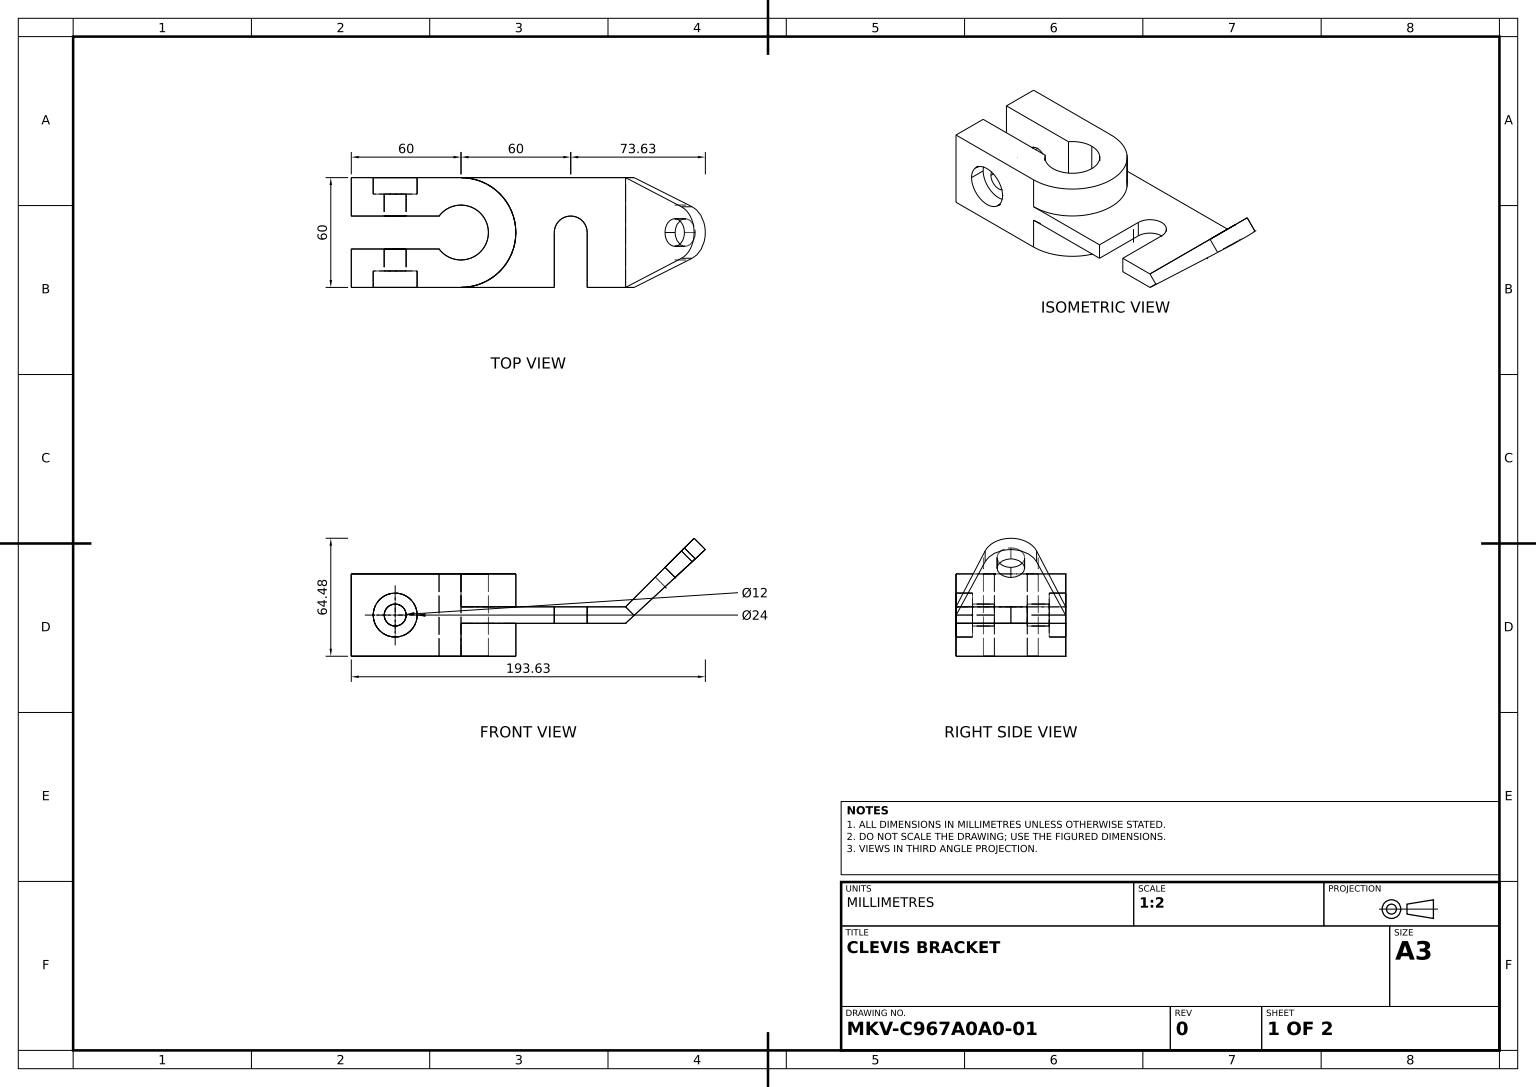
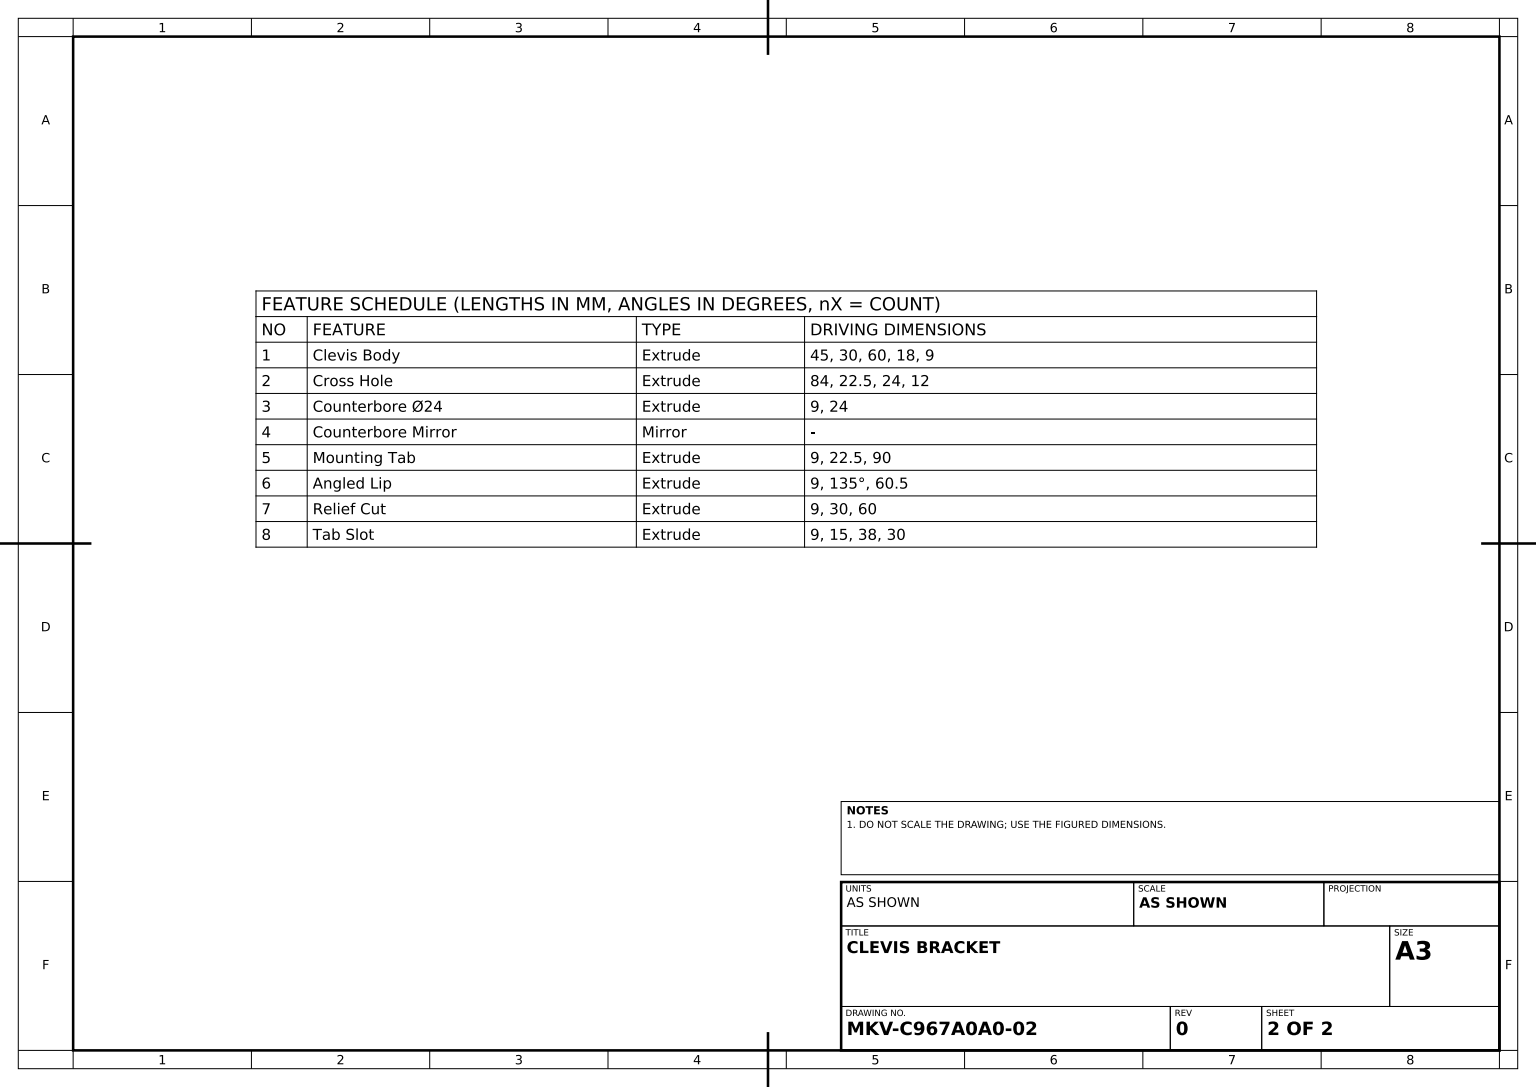
SolidWorks part; units mm, degrees
material "Plain Carbon Steel"
ref_plane "Front Plane" through (0, 0, 0) normal (0, 0, 1) x (1, 0, 0)
ref_plane "Top Plane" through (0, 0, 0) normal (0, 1, 0) x (1, 0, 0)
ref_plane "Right Plane" through (0, 0, 0) normal (1, 0, 0) x (0, 0, -1)
sketch "Clevis Body Sketch" plane through (0, 0, 0) normal (0, 1, 0) x (1, 0, 0)
  line L0 (87.3027, 0) -> (-87.3027, 0) construction
  line L1 (-12, 9) -> (-60, 9)
  line L3 (-60, -9) -> (-12, -9)
  line L4 (0, 30) -> (-60, 30)
  line L5 (-60, 30) -> (-60, 9)
  line L6 (-60, -9) -> (-60, -30)
  line L7 (-60, -30) -> (0, -30)
  arc A0 (-12, -9) -> (-12, 9) centre (0, 0) ccw
  arc A1 (0, -30) -> (0, 30) centre (0, 0) ccw
  point P6 (0, 0)
  point P12 (0, 0)
  dimension "D1" = 30
  dimension "D2" = 60
  dimension "D3" = 18
  dimension "D4" = 9
  dimension "D5" = 60
  dimension "D6" = 9
extrude "Clevis Body" add sketch "Clevis Body Sketch" along normal mid plane 45
sketch "Cross Hole Sketch" plane through (0, 0, 30) normal (0, 0, 1) x (1, 0, 0)
  line L0 (-60, -22.5) -> (0, -22.5) construction
  line L1 (-60, 22.5) -> (-60, -22.5) construction
  circle A0 centre (-36, 0) radius 6
  dimension "D3" = 12
  dimension "D1" = 22.5
  dimension "D2" = 24
extrude "Cross Hole" cut sketch "Cross Hole Sketch" against normal blind 84
sketch "Counterbore Sketch" plane through (0, 0, 30) normal (0, 0, 1) x (1, 0, 0)
  circle A0 centre (-36, 0) radius 12
  dimension "D1" = 24
extrude "Counterbore Ø24" cut sketch "Counterbore Sketch" against normal blind 9
mirror "Counterbore Mirror" about plane through (0, 0, 0) normal (0, 0, 1) of "Counterbore Ø24"
sketch "Mounting Tab Sketch" plane through (0, 22.5, 0) normal (0, 1, 0) x (1, 0, 0)
  line L0 (0, 30) -> (90, 30)
  line L1 (90, 30) -> (90, -30)
  line L2 (90, -30) -> (0, -30)
  arc A0 (0, -30) -> (0, 30) centre (0, 0) ccw construction
  arc A1 (0, -30) -> (0, 30) centre (0, 0) ccw
  dimension "D1" = 90
extrude "Mounting Tab" add sketch "Mounting Tab Sketch" against normal mid plane 9 from offset 22.5 offset against normal yes
sketch "Angled Lip Sketch" plane through (0, 0, 30) normal (0, 0, 1) x (1, 0, 0)
  line L0 (90, -4.5) -> (90, 4.5) construction
  line L1 (90, -4.5) -> (90, 4.5)
  line L2 (90, 4.5) -> (132.78, 47.28)
  line L3 (132.78, 47.28) -> (139.1439, 40.916)
  line L4 (139.1439, 40.916) -> (90, -4.5)
  line L5 (0, 4.5) -> (90, 4.5) construction
  dimension "D1" = 9
  dimension "D2" = 135
  dimension "D3" = 60.5
extrude "Angled Lip" add sketch "Angled Lip Sketch" against normal up to surface (60 mm away) up to face at (-24, 0, -30)
sketch "Relief Cut Sketch" plane through (0, 4.5, 0) normal (0, 1, 0) x (1, 0, 0)
  line L0 (51, -30) -> (51, 0)
  line L1 (0, -30) -> (90, -30) construction
  line L2 (69, 0) -> (69, -30)
  line L3 (69, -30) -> (51, -30)
  line L4 (90, 30) -> (0, 30) construction
  arc A0 (51, 0) -> (69, 0) centre (60, 0) cw
  point P9 (60, -30)
  dimension "D1" = 9
  dimension "D2" = 30
  dimension "D3" = 60
extrude "Relief Cut" cut sketch "Relief Cut Sketch" against normal blind 9
sketch "Tab Slot Sketch" plane through (42.75, -42.75, 0) normal (-0.7071, 0.7071, 0) x (0, 0, 1)
  line L0 (30, 66.8216) -> (-30, 66.8216) construction
  line L1 (-30, 66.8216) -> (-14.0736, 110.0113)
  line L2 (30, 66.8216) -> (14.0736, 110.0113)
  line L3 (-30, 66.8216) -> (-30, 127.3216)
  line L4 (-30, 127.3216) -> (30, 127.3216)
  line L5 (30, 127.3216) -> (30, 66.8216)
  circle A0 centre (0, 104.8216) radius 7.5
  arc A1 (14.0736, 110.0113) -> (-14.0736, 110.0113) centre (0, 104.8216) ccw
  dimension "D1" = 15
  dimension "D3" = 30
  dimension "D2" = 38
extrude "Tab Slot" cut sketch "Tab Slot Sketch" against normal blind 9
